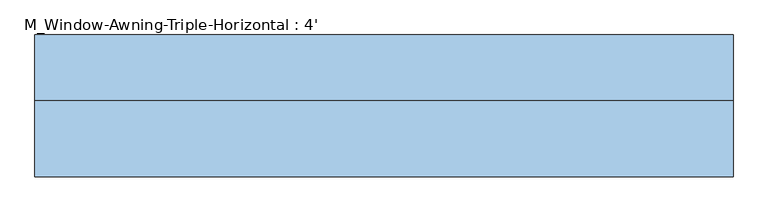
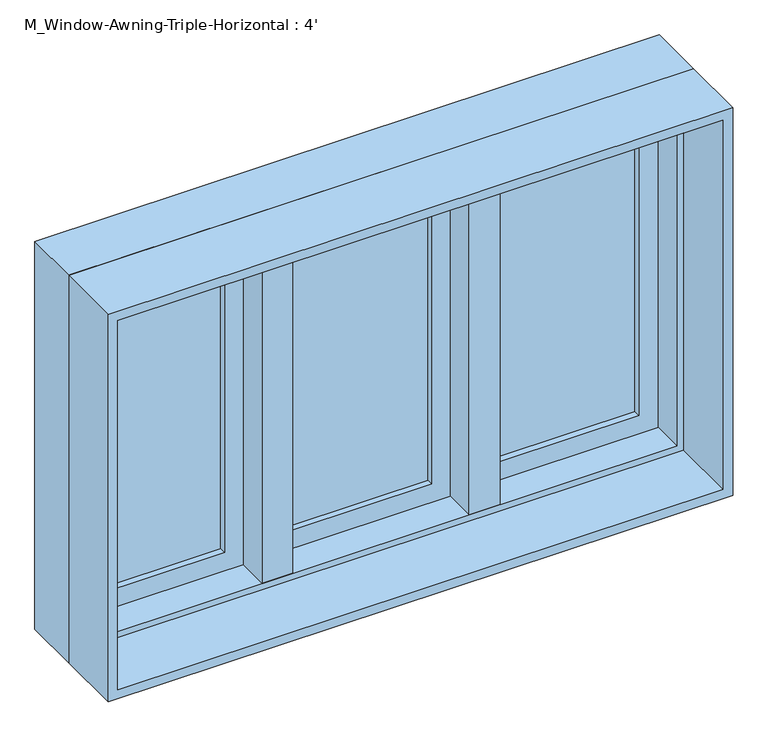
"""IFC4 building model written with IfcOpenShell, lengths in millimetres: window geometry, M_Window-Awning-Triple-Horizontal : 4'."""

from ifc_helpers import new_model, si_unit, frame, origin, place, context, project, spatial, polyline, outline, extrude, faceted_brep, source, transform, mapped, element, save


def m_window_awning_triple_horizontal_4_d9bc2bdd(model_context):
    return source(origin(), model_context, "Body", "SolidModel", [
        faceted_brep([(577.85, 82.55, 1668.25), (577.85, 19.05, 1668.25), (-577.85, 19.05, 1668.25), (-577.85, 82.55, 1668.25), (596.9, 133.35, 1687.3), (596.9, 82.55, 1687.3), (-596.9, 82.55, 1687.3), (-596.9, 133.35, 1687.3), (609.6, 19.05, 1700.0), (609.6, 133.35, 1700.0), (-609.6, 133.35, 1700.0), (-609.6, 19.05, 1700.0), (-577.85, 19.05, 931.75), (-577.85, 82.55, 931.75), (-596.9, 82.55, 912.7), (-596.9, 133.35, 912.7), (-609.6, 133.35, 900.0), (-609.6, 19.05, 900.0), (577.85, 19.05, 931.75), (577.85, 82.55, 931.75), (596.9, 82.55, 912.7), (596.9, 133.35, 912.7), (609.6, 133.35, 900.0), (609.6, 19.05, 900.0)], [[[0, 1, 2, 3]], [[4, 5, 6, 7]], [[8, 9, 10, 11]], [[3, 2, 12, 13]], [[7, 6, 14, 15]], [[11, 10, 16, 17]], [[13, 12, 18, 19]], [[15, 14, 20, 21]], [[17, 16, 22, 23]], [[11, 17, 23, 8], [1, 18, 12, 2]], [[19, 18, 1, 0]], [[5, 20, 14, 6], [3, 13, 19, 0]], [[21, 20, 5, 4]], [[23, 22, 9, 8]], [[9, 22, 16, 10], [7, 15, 21, 4]]]),
        extrude(outline(polyline([(1700.0, -609.6), (900.0, -609.6), (900.0, 609.6), (1700.0, 609.6), (1700.0, -609.6)]), holes=[polyline([(1680.95, 590.55), (919.05, 590.55), (919.05, -590.55), (1680.95, -590.55), (1680.95, 590.55)])]), frame((0.0, -114.3, 0.0), z_axis=(0.0, 1.0, 0.0), x_axis=(0.0, 0.0, 1.0)), (0.0, 0.0, 1.0), 133.35),
        extrude(outline(polyline([(912.7, 596.9), (1687.3, 596.9), (1687.3, 211.6666667), (912.7, 211.6666667), (912.7, 596.9)]), holes=[polyline([(969.85, 268.8166667), (1630.15, 268.8166667), (1630.15, 539.75), (969.85, 539.75), (969.85, 268.8166667)])]), frame((0.0, 82.55, 0.0), z_axis=(0.0, 1.0, 0.0), x_axis=(0.0, 0.0, 1.0)), (0.0, 0.0, 1.0), 44.45),
        extrude(outline(polyline([(1687.3, -596.9), (912.7, -596.9), (912.7, -211.6666667), (1687.3, -211.6666667), (1687.3, -596.9)]), holes=[polyline([(1630.15, -268.8166667), (969.85, -268.8166667), (969.85, -539.75), (1630.15, -539.75), (1630.15, -268.8166667)])]), frame((0.0, 82.55, 0.0), z_axis=(0.0, 1.0, 0.0), x_axis=(0.0, 0.0, 1.0)), (0.0, 0.0, 1.0), 44.45),
        extrude(outline(polyline([(539.75, 114.3), (539.75, 107.95), (268.8166667, 107.95), (268.8166667, 114.3), (539.75, 114.3)])), frame((0.0, 0.0, 969.85), z_axis=(0.0, 0.0, 1.0), x_axis=(1.0, 0.0, 0.0)), (0.0, 0.0, 1.0), 660.3),
        extrude(outline(polyline([(268.8166667, 95.25), (268.8166667, 101.6), (539.75, 101.6), (539.75, 95.25), (268.8166667, 95.25)])), frame((0.0, 0.0, 969.85), z_axis=(0.0, 0.0, 1.0), x_axis=(1.0, 0.0, 0.0)), (0.0, 0.0, 1.0), 660.3),
        extrude(outline(polyline([(-268.8166667, 114.3), (-268.8166667, 107.95), (-539.75, 107.95), (-539.75, 114.3), (-268.8166667, 114.3)])), frame((0.0, 0.0, 969.85), z_axis=(0.0, 0.0, 1.0), x_axis=(1.0, 0.0, 0.0)), (0.0, 0.0, 1.0), 660.3),
        extrude(outline(polyline([(-539.75, 95.25), (-539.75, 101.6), (-268.8166667, 101.6), (-268.8166667, 95.25), (-539.75, 95.25)])), frame((0.0, 0.0, 969.85), z_axis=(0.0, 0.0, 1.0), x_axis=(1.0, 0.0, 0.0)), (0.0, 0.0, 1.0), 660.3),
        extrude(outline(polyline([(135.4666667, 114.3), (135.4666667, 107.95), (-135.4666667, 107.95), (-135.4666667, 114.3), (135.4666667, 114.3)])), frame((0.0, 0.0, 969.85), z_axis=(0.0, 0.0, 1.0), x_axis=(1.0, 0.0, 0.0)), (0.0, 0.0, 1.0), 660.3),
        extrude(outline(polyline([(-135.4666667, 95.25), (-135.4666667, 101.6), (135.4666667, 101.6), (135.4666667, 95.25), (-135.4666667, 95.25)])), frame((0.0, 0.0, 969.85), z_axis=(0.0, 0.0, 1.0), x_axis=(1.0, 0.0, 0.0)), (0.0, 0.0, 1.0), 660.3),
        extrude(outline(polyline([(912.7, 192.6166667), (1687.3, 192.6166667), (1687.3, -192.6166667), (912.7, -192.6166667), (912.7, 192.6166667)]), holes=[polyline([(969.85, -135.4666667), (1630.15, -135.4666667), (1630.15, 135.4666667), (969.85, 135.4666667), (969.85, -135.4666667)])]), frame((0.0, 82.55, 0.0), z_axis=(0.0, 1.0, 0.0), x_axis=(0.0, 0.0, 1.0)), (0.0, 0.0, 1.0), 44.45),
        faceted_brep([(192.6166667, 82.55, 1687.3), (172.1065328, 82.55, 1687.3), (172.1065328, 19.05, 1687.3), (232.1768005, 19.05, 1687.3), (232.1768005, 82.55, 1687.3), (211.6666667, 82.55, 1687.3), (211.6666667, 133.35, 1687.3), (192.6166667, 133.35, 1687.3), (192.6166667, 133.35, 912.7), (211.6666667, 133.35, 912.7), (211.6666667, 104.775, 912.7), (192.6166667, 104.775, 912.7), (192.6166667, 82.55, 1680.95), (172.1065328, 82.55, 1680.95), (192.6166667, 82.55, 1668.25), (192.6166667, 82.55, 931.75), (172.1065328, 82.55, 931.75), (172.1065328, 82.55, 1668.25), (172.1065328, 19.05, 1680.95), (172.1065328, 19.05, 931.75), (172.1065328, 19.05, 1668.25), (232.1768005, 19.05, 1680.95), (232.1768005, 19.05, 931.75), (232.1768005, 19.05, 1668.25), (232.1768005, 82.55, 1680.95), (232.1768005, 82.55, 931.75), (232.1768005, 82.55, 1668.25), (211.6666667, 82.55, 1680.95), (211.6666667, 82.55, 931.75), (211.6666667, 82.55, 1668.25), (211.6666667, 104.775, 1680.95), (211.6666667, 104.775, 1668.25), (211.6666667, 104.775, 931.75), (192.6166667, 104.775, 931.75), (192.6166667, 104.775, 1668.25), (192.6166667, 104.775, 1680.95)], [[[0, 1, 2, 3, 4, 5, 6, 7]], [[8, 9, 10, 11]], [[1, 0, 12, 13]], [[14, 15, 16, 17]], [[2, 1, 13, 18]], [[17, 16, 19, 20]], [[3, 2, 18, 21]], [[20, 19, 22, 23]], [[4, 3, 21, 24]], [[23, 22, 25, 26]], [[5, 4, 24, 27]], [[26, 25, 28, 29]], [[6, 5, 27, 30, 31, 29, 28, 32, 10, 9]], [[0, 7, 8, 11, 33, 15, 14, 34, 35, 12]], [[30, 35, 34, 31]], [[32, 33, 11, 10]], [[35, 30, 27, 24, 21, 18, 13, 12]], [[31, 34, 14, 17, 20, 23, 26, 29]], [[33, 32, 28, 25, 22, 19, 16, 15]], [[7, 6, 9, 8]]]),
        faceted_brep([(-211.6666667, 82.55, 1687.3), (-232.1768005, 82.55, 1687.3), (-232.1768005, 19.05, 1687.3), (-172.1065328, 19.05, 1687.3), (-172.1065328, 82.55, 1687.3), (-192.6166667, 82.55, 1687.3), (-192.6166667, 133.35, 1687.3), (-211.6666667, 133.35, 1687.3), (-211.6666667, 133.35, 912.7), (-192.6166667, 133.35, 912.7), (-192.6166667, 104.775, 912.7), (-211.6666667, 104.775, 912.7), (-232.1768005, 82.55, 1680.95), (-232.1768005, 19.05, 1680.95), (-232.1768005, 82.55, 1668.25), (-232.1768005, 82.55, 931.75), (-232.1768005, 19.05, 931.75), (-232.1768005, 19.05, 1668.25), (-172.1065328, 19.05, 1680.95), (-172.1065328, 19.05, 931.75), (-172.1065328, 19.05, 1668.25), (-172.1065328, 82.55, 1680.95), (-172.1065328, 82.55, 931.75), (-172.1065328, 82.55, 1668.25), (-192.6166667, 82.55, 1680.95), (-192.6166667, 104.775, 1680.95), (-192.6166667, 104.775, 1668.25), (-192.6166667, 82.55, 1668.25), (-192.6166667, 82.55, 931.75), (-192.6166667, 104.775, 931.75), (-211.6666667, 104.775, 931.75), (-211.6666667, 82.55, 931.75), (-211.6666667, 82.55, 1668.25), (-211.6666667, 104.775, 1668.25), (-211.6666667, 104.775, 1680.95), (-211.6666667, 82.55, 1680.95)], [[[0, 1, 2, 3, 4, 5, 6, 7]], [[8, 9, 10, 11]], [[2, 1, 12, 13]], [[14, 15, 16, 17]], [[3, 2, 13, 18]], [[17, 16, 19, 20]], [[4, 3, 18, 21]], [[20, 19, 22, 23]], [[6, 5, 24, 25, 26, 27, 28, 29, 10, 9]], [[0, 7, 8, 11, 30, 31, 32, 33, 34, 35]], [[25, 34, 33, 26]], [[29, 30, 11, 10]], [[34, 25, 24, 21, 18, 13, 12, 35]], [[26, 33, 32, 14, 17, 20, 23, 27]], [[30, 29, 28, 22, 19, 16, 15, 31]], [[1, 0, 35, 12]], [[15, 14, 32, 31]], [[5, 4, 21, 24]], [[28, 27, 23, 22]], [[7, 6, 9, 8]]]),
    ])


if __name__ == "__main__":
    model = new_model("IFC4")
    model_context = context("Model", 3, world=origin())
    ifc_project = project(units=[si_unit("LENGTHUNIT", "METRE", prefix="MILLI")], contexts=[model_context])
    site = spatial("IfcSite", under=ifc_project)
    building = spatial("IfcBuilding", under=site)
    placement = place(None, origin())
    m_window_awning_triple_horizontal_4_shape = m_window_awning_triple_horizontal_4_d9bc2bdd(model_context)
    element("IfcWindow", 1, ObjectType="M_Window-Awning-Triple-Horizontal : 4'", at=placement, inside=building, context=model_context, shape_type="MappedRepresentation", body=[
        mapped(m_window_awning_triple_horizontal_4_shape, transform((0.0, 0.0, 0.0), x_axis=(1.0, 0.0, 0.0), y_axis=(0.0, 1.0, 0.0), z_axis=(0.0, 0.0, 1.0))),
    ])
    save(model, "model.ifc")

# Revit data of these elements
# Type "M_Window-Awning-Triple-Horizontal : 4'"
#   Type Mark = "19"
#   Fire Rating = "0.5h"
#   Assembly Code = "B2020100"
#   Analytic Construction = "Double glazing - domestic"
#   Window Inset [instance default] = 0' - 0"
#   Wall Thickness [instance default] = 0' - 5.90551"
#   Muntin Width = 0' - 10.66667"
#   Visual Light Transmittance = 0.81
#   Thermal Resistance (R) = 1.8146 (h·ft²·°F)/BTU
#   Solar Heat Gain Coefficient = 0.76
#   One Third Width = 1' - 4"
#   Sash Width = 1' - 3.16667"
#   Rough Width = 4' - 0.59055"
#   Rough Height = 2' - 8.08661"
#   Interior Wall Closure [instance default] = 0' - 2.15551"
#   Height = 2' - 7.49606"
#   Heat Transfer Coefficient (U) = 0.5511 BTU/(h·ft²·°F)
#   Muntin Height = 2' - 1.99606"
#   Frame Extension [instance default] = 0' - 0 1/4"
#   Exterior Wall Closure [instance default] = 0' - 1 1/4"
#   Extension Jamb [instance default] = 0' - 2.15551"
#   Default Sill Height = 2' - 11.43307"
#   Width = 4' - 0"
#   Middle Muntin Visibility = yes
#   Side Muntin Visibility = yes
#   Interior Trim Visibility [instance default] = yes
#   Exterior Trim Visibility [instance default] = yes
#   Extension Jamb Visibility [instance default] = yes
#   Muntin Pattern = M_Muntin Pattern_2x2 : M_Muntin Pattern_2x2
#   Interior Trim Material = Wood - Stained
#   Interior Trim = M_Trim-Window-Interior-Flat : Picture Frame
#   Interior Frame Material = Wood - Stained
#   Glass Panel Material = Glass
#   Exterior Trim Material = Clad - White
#   Exterior Trim = M_Trim-Window-Exterior-Flat : with Sill
#   Exterior Frame Material = Clad - White
#   Wall Closure = (empty or 0)
# Element 1 (IfcWindow, "M_Window-Awning-Triple-Horizontal : 4'")
#   Wall Thickness = 0' - 9"
#   Extension Jamb = 0' - 5 1/4"
#   Materials on its faces: "Wood - Stained", "Glass", "Clad - White"
# Materials
#   "Wood - Stained": class "Wood", colour RGB 224 178 126, transparency 0, Cost = 0
#   "Glass": class "Glass", colour RGB 0 128 192, transparency 0.75, Description = "Soda Lime Glass", Cost = 0
#   "Clad - White": class "Wood", colour RGB 242 242 238, transparency 0, Cost = 0
